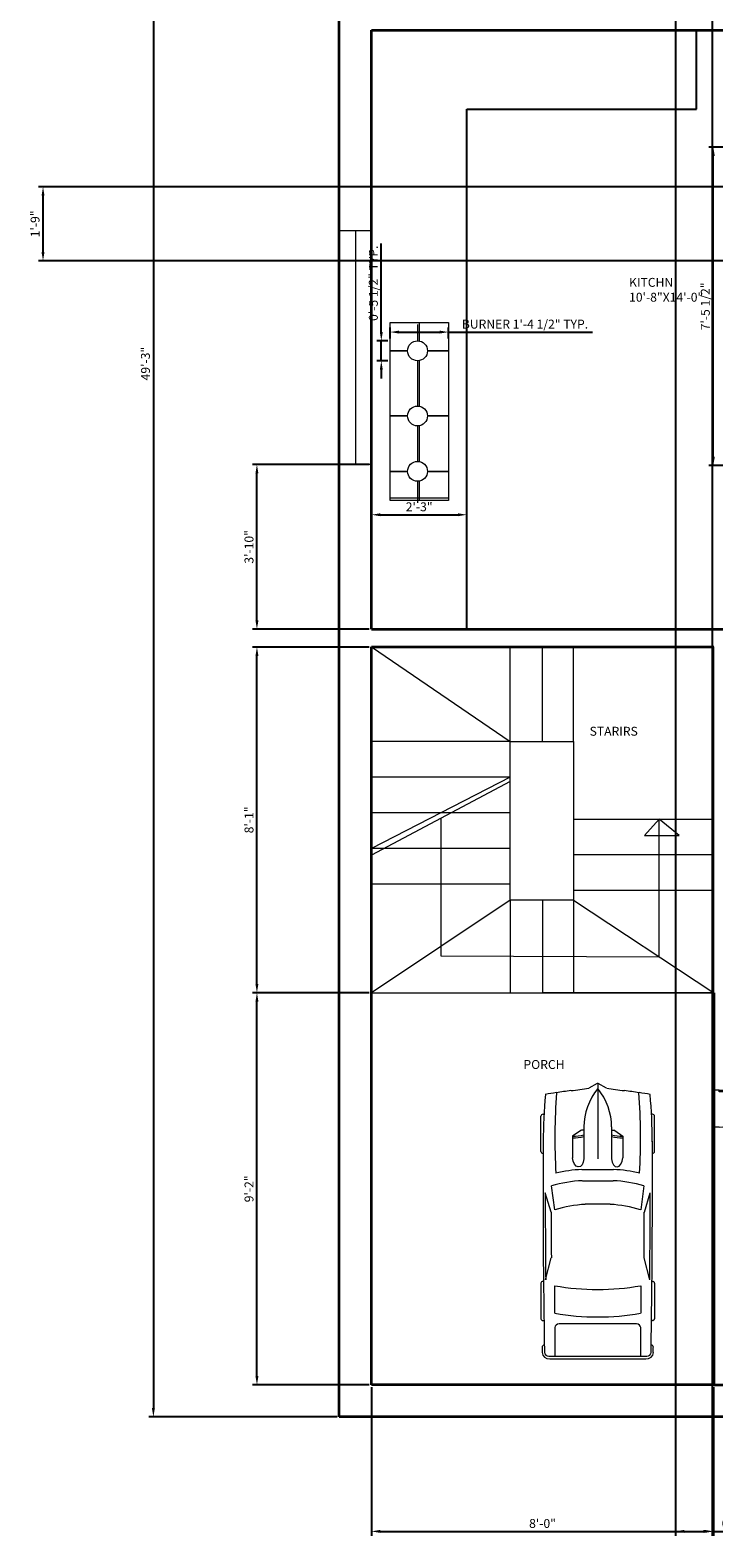
# Model space of a CAD drawing. Units: inches. Extents: x 311 to 793, y -3602 to -2932.
# Tile 1 of 3: x 313 to 505, y -3602 to -3179. Entities that reach past the tile are written whole.
import ezdxf

# ---------------------------------------------------------------- set-up
doc = ezdxf.new("R2010")
doc.units = ezdxf.units.IN
for name, color, linetype, lineweight in [('A-ANNO-DIMS', 2, 'Continuous', 18), ('A-AREA-IDEN', 7, 'Continuous', 18), ('A-DOOR', 3, 'Continuous', 18), ('A-EQPM', 9, 'Continuous', 18), ('A-FLOR-CASE', 9, 'Continuous', 25), ('A-FLOR-STRS', 7, 'Continuous', 18), ('A-GLAZ', 4, 'Continuous', 18), ('A-SITE-VEHC', 8, 'Continuous', 13), ('A-WALL', 7, 'Continuous', 35)]:
    doc.layers.add(name, color=color, linetype=linetype, lineweight=lineweight)
doc.styles.get("Standard").update_dxf_attribs({"font": 'arial.ttf'})
doc.dimstyles.new('ISO-25', dxfattribs={"dimtxt": 2.5, "dimasz": 2.5, "dimexe": 1.25, "dimexo": 0.625, "dimtad": 1, "dimlunit": 3, "dimtxsty": 'Standard', "dimcen": 2.5, "dimadec": 0, "dimazin": 0, "dimtfac": 1, "dimtmove": 0, "dimatfit": 3, "dimfxl": 1, "dimarcsym": 0})

# ---------------------------------------------------------------- blocks, each defined once
blk = doc.blocks.new('*U2')
for p, q in [((0, 0), (0, -6)), ((40, 0), (40, -6))]:
    blk.add_line(p, q)
blk.add_lwpolyline([(0, 0), (0, 40), (1.75, 40), (1.75, 0)], close=True)
blk.add_arc((0, 0), 40, 0, 90)
blk = doc.blocks.new('*U10')
for p, q in [((21.1, 37.4), (21.1, 36.8)), ((46.6, 38.9), (22.4, 38.9)), ((47.8, 37.4), (47.8, 37.4)), ((70, 31.5), (86.4, 29.4)), ((88, 31.9), (74.8, 35.9)), ((134.3, 35.6), (119.3, 31.8)), ((135.5, 37.1), (135.5, 37.4)), ((136.7, 38.9), (160.9, 38.9)), ((162.1, 37.4), (162.1, 36.8)), ((186.5, -33.5), (186.5, 33.5)), ((188.4, -32.8), (188.4, 32.8)), ((138.4, 29.4), (157.2, 29.4)), ((164.5, 26.4), (164.5, -26.4)), ((186.5, 29.4), (167, 29.4)), ((32.1, 9.5), (32.1, 11.2)), ((32.3, 11.6), (36.1, 17.2)), ((36.1, 17.2), (50.9, 17.2)), ((58.9, -10.8), (58.9, 10.8)), ((66.6, -10.5), (66.6, 10.5)), ((186.5, -10.5), (186.5, 10.5)), ((3.3, 6.1), (0.1, 0.4)), ((29.8, 9.5), (51.7, 9.5)), ((82.7, 8.5), (82.7, -8.5)), ((0, 0), (51.7, 0)), ((0.1, -0.4), (3.3, -6.1)), ((29.8, -9.5), (51.7, -9.5)), ((32.1, -9.5), (32.1, -11.2)), ((32.3, -11.6), (36.1, -17.2)), ((36.1, -17.2), (50.9, -17.2)), ((86.4, -29.4), (70, -31.5)), ((157.2, -29.4), (138.4, -29.4)), ((167, -29.4), (186.5, -29.4)), ((21.1, -37.4), (21.1, -36.8)), ((46.6, -38.9), (22.4, -38.9)), ((47.8, -37.4), (47.8, -37.4)), ((88, -31.9), (74.8, -35.9)), ((134.3, -35.6), (119.3, -31.8)), ((135.5, -37.1), (135.5, -37.4)), ((136.7, -38.9), (160.9, -38.9)), ((162.1, -37.4), (162.1, -36.8))]:
    blk.add_line(p, q)
for centre, major_axis, ratio, start_param, end_param in [((266, -27.5), (0, 313.3), 0.842304, 1.367076, 1.39176), ((41.2, -490.9), (0, 528.2), 0.842304, 0.00281, 0.075598), ((22.4, 37.4), (0, -1.48), 0.842304, 3.141593, 4.712389), ((64.5, -10555.6), (0, 10593), 0.842304, -0.013397, 0.002797), ((46.6, 37.4), (0, 1.48), 0.842304, -1.570796, 0), ((135.3, 5.4), (0, 81.8), 0.842304, 1.245306, 1.50788), ((64.5, -10555.6), (0, -10591.5), 0.842304, 3.133765, 3.140441), ((95.8, -3666.4), (0, -3698.2), 0.842304, 3.134049, 3.144098), ((136.7, 37.4), (0, -1.48), 0.842304, 3.141593, 4.712389), ((160.9, 37.4), (0, 1.48), 0.842304, -1.570796, 0), ((180.6, 35.8), (0, 2.22), 0.842304, -0.013017, 1.249894), ((64.5, -10556.4), (0, 10595.3), 0.842304, -0.013397, -0.013017), ((184, 32.8), (0, -5.25), 0.842304, 1.570796, 3.128196), ((184, 33.5), (0, -2.96), 0.842304, 1.570796, 3.128196), ((259.2, -27.5), (0, -305.3), 0.842304, 4.528606, 4.561838), ((37.5, -594), (0, -623.3), 0.842304, 3.096046, 3.200911), ((134.4, 5.4), (0, -89.8), 0.842304, 4.449482, 4.652344), ((149.6, 2.8), (0, -79.6), 0.842304, 4.372215, 4.640744), ((17.1, 0), (0, 147), 0.842304, 4.511394, 4.913384), ((35.9, 0), (0, 147), 0.842304, 4.511394, 4.913384), ((167, 26.4), (0, 2.96), 0.842304, 0, 1.570796), ((-204.5, 52.4), (0, -251), 0.842304, 1.385369, 1.434372), ((32.7, 11.2), (0, 0.74), 0.842304, 0.879714, 1.570796), ((13, 17), (0, 27.4), 0.842304, 4.435146, 4.718221), ((14.2, 17), (0, 27.4), 0.842304, 4.435146, 4.718221), ((50.8, 13.3), (6.34, -0.36), 0.603834, -1.395552, 1.581315), ((0.6, 0), (0, -0.74), 0.842304, 4.131459, 5.293319), ((29.8, -46.7), (0, 56.2), 0.842304, 0, 0.590319), ((-204.5, -52.4), (0, 251), 0.842304, -1.434372, -1.385369), ((29.8, 46.7), (0, 56.2), 0.842304, 2.551274, 3.141593), ((13, -17), (0, -27.4), 0.842304, 1.564964, 1.848039), ((14.2, -17), (0, -27.4), 0.842304, 1.564964, 1.848039), ((149.6, -2.8), (0, -79.6), 0.842304, -1.499151, -1.230623), ((259.2, 27.5), (0, 305.3), 0.842304, 1.721348, 1.754579), ((32.7, -11.2), (0, -0.74), 0.842304, 4.712389, 5.403472), ((134.4, -5.4), (0, -89.8), 0.842304, -1.510751, -1.307889), ((135.3, -5.4), (0, -81.8), 0.842304, -1.50788, -1.245306), ((266, 27.5), (0, 313.3), 0.842304, 1.749832, 1.774517), ((37.5, 594), (0, -623.3), 0.842304, -0.059319, 0.045547), ((167, -26.4), (0, -2.96), 0.842304, 4.712389, 6.283185), ((41.2, 490.9), (0, -528.2), 0.842304, -0.075598, -0.00281), ((22.4, -37.4), (0, 1.48), 0.842304, 1.570796, 3.141593), ((64.5, 10555.6), (0, 10593), 0.842304, 3.138796, 3.15499), ((46.6, -37.4), (0, -1.48), 0.842304, 0, 1.570796), ((64.5, 10555.6), (0, -10591.5), 0.842304, 0.001152, 0.007828), ((95.8, 3666.4), (0, -3698.2), 0.842304, -0.002505, 0.007544), ((136.7, -37.4), (0, -1.48), 0.842304, -1.570796, 0), ((160.9, -37.4), (0, 1.48), 0.842304, 3.141593, 4.712389), ((180.6, -35.8), (0, -2.22), 0.842304, -1.249894, 0.013017), ((64.5, 10556.4), (0, 10595.3), 0.842304, 3.15461, 3.15499), ((184, -32.8), (0, -5.25), 0.842304, 0.013397, 1.570796), ((184, -33.5), (0, 2.96), 0.842304, 3.15499, 4.712389)]:
    blk.add_ellipse(centre, major_axis=major_axis, ratio=ratio, start_param=start_param, end_param=end_param)
at = {"extrusion": (0, 0, -1)}
blk.add_ellipse((50.8, -13.3), major_axis=(6.34, 0.36), ratio=0.603834, start_param=-1.395552, end_param=1.581315, dxfattribs=at)
blk = doc.blocks.new('*D12')
at = {"layer": 'A-ANNO-DIMS', "color": 0, "lineweight": -2, "transparency": 16777216}
for p, q in [((399.17, -2976.63), (346.4, -2976.63)), ((347.65, -2979.13), (347.65, -3565.13)), ((399.17, -3567.63), (346.4, -3567.63))]:
    blk.add_line(p, q, dxfattribs=at)
at = {"layer": 'A-ANNO-DIMS', "color": 0, "transparency": 16777216}
for points in [[(347.23, -2979.13), (348.07, -2979.13), (347.65, -2976.63)], [(347.23, -3565.13), (348.07, -3565.13), (347.65, -3567.63)]]:
    blk.add_solid(points, dxfattribs=at)
at = {"layer": 'Defpoints', "color": 0, "transparency": 16777216}
for p in [(399.79, -2976.63), (347.65, -3567.63), (399.79, -3567.63)]:
    blk.add_point(p, dxfattribs=at)
at = {"layer": 'A-ANNO-DIMS', "color": 0, "transparency": 16777216, "insert": (345.75, -3272.13), "char_height": 2.5, "attachment_point": 5, "rotation": 90}
blk.add_mtext('49\'-3"', dxfattribs=at)
blk = doc.blocks.new('WINDOW-SIDE-66')
for p, q in [((0, 65.66), (9, 65.66)), ((0, 0), (0, 65.66)), ((0, 65.66), (4.5, 65.66)), ((4.5, 65.66), (4.5, 0)), ((9, 65.66), (9, 0)), ((9, 0), (0, 0))]:
    blk.add_line(p, q)
blk = doc.blocks.new('COOKTOP-BURNER')
for p, q in [((4.91, 2.79), (0, 2.79)), ((4.91, 2.69), (0, 2.69)), ((16.38, 2.79), (10.5, 2.79)), ((10.5, 2.79), (16.38, 2.79)), ((16.38, 2.69), (10.5, 2.69))]:
    blk.add_line(p, q)
blk.add_circle((7.71, 2.79), 2.79)
blk = doc.blocks.new('*D20')
at = {"layer": 'A-ANNO-DIMS', "color": 0, "lineweight": -2, "transparency": 16777216}
for p, q in [((414.03, -3265.11), (414.03, -3262.03)), ((416.53, -3263.28), (427.91, -3263.28)), ((430.41, -3265.11), (430.41, -3262.03)), ((430.41, -3263.28), (470.83, -3263.28))]:
    blk.add_line(p, q, dxfattribs=at)
at = {"layer": 'A-ANNO-DIMS', "color": 0, "transparency": 16777216}
for points in [[(416.53, -3262.87), (416.53, -3263.7), (414.03, -3263.28)], [(427.91, -3262.87), (427.91, -3263.7), (430.41, -3263.28)]]:
    blk.add_solid(points, dxfattribs=at)
at = {"layer": 'Defpoints', "color": 0, "transparency": 16777216}
for p in [(430.41, -3263.28), (414.03, -3265.74), (430.41, -3265.74)]:
    blk.add_point(p, dxfattribs=at)
at = {"layer": 'A-ANNO-DIMS', "color": 0, "transparency": 16777216, "insert": (451.87, -3261.37), "char_height": 2.5, "attachment_point": 5}
blk.add_mtext('BURNER 1\'-4 1/2" TYP.', dxfattribs=at)
blk = doc.blocks.new('*D21')
at = {"layer": 'A-ANNO-DIMS', "color": 0, "lineweight": -2, "transparency": 16777216}
for p, q in [((411.57, -3263.24), (411.57, -3238.43)), ((413.4, -3265.74), (410.32, -3265.74)), ((411.57, -3271.32), (411.57, -3265.74)), ((413.4, -3271.32), (410.32, -3271.32)), ((411.57, -3273.82), (411.57, -3276.32))]:
    blk.add_line(p, q, dxfattribs=at)
at = {"layer": 'A-ANNO-DIMS', "color": 0, "transparency": 16777216}
for points in [[(411.16, -3263.24), (411.99, -3263.24), (411.57, -3265.74)], [(411.16, -3273.82), (411.99, -3273.82), (411.57, -3271.32)]]:
    blk.add_solid(points, dxfattribs=at)
at = {"layer": 'Defpoints', "color": 0, "transparency": 16777216}
for p in [(411.57, -3265.74), (414.03, -3265.74), (414.03, -3271.32)]:
    blk.add_point(p, dxfattribs=at)
at = {"layer": 'A-ANNO-DIMS', "color": 0, "transparency": 16777216, "insert": (409.66, -3249.58), "char_height": 2.5, "attachment_point": 5, "rotation": 90}
blk.add_mtext('0\'-5 1/2" TYP.', dxfattribs=at)
blk = doc.blocks.new('*D25')
at = {"layer": 'A-ANNO-DIMS', "color": 0, "lineweight": -2, "transparency": 16777216}
for p, q in [((408.79, -3559.25), (408.79, -3600.98)), ((504.79, -3559.25), (504.79, -3600.98)), ((411.29, -3599.73), (502.29, -3599.73))]:
    blk.add_line(p, q, dxfattribs=at)
at = {"layer": 'A-ANNO-DIMS', "color": 0, "transparency": 16777216}
for points in [[(411.29, -3599.31), (411.29, -3600.14), (408.79, -3599.73)], [(502.29, -3599.31), (502.29, -3600.14), (504.79, -3599.73)]]:
    blk.add_solid(points, dxfattribs=at)
at = {"layer": 'Defpoints', "color": 0, "transparency": 16777216}
for p in [(408.79, -3558.63), (504.79, -3558.63), (504.79, -3599.73)]:
    blk.add_point(p, dxfattribs=at)
at = {"layer": 'A-ANNO-DIMS', "color": 0, "transparency": 16777216, "insert": (456.79, -3597.82), "char_height": 2.5, "attachment_point": 5}
blk.add_mtext('8\'-0"', dxfattribs=at)
blk = doc.blocks.new('*D32')
at = {"layer": 'A-ANNO-DIMS', "color": 0, "lineweight": -2, "transparency": 16777216}
for p, q in [((408.17, -3448.63), (375.44, -3448.63)), ((376.69, -3556.13), (376.69, -3451.13)), ((408.17, -3558.63), (375.44, -3558.63))]:
    blk.add_line(p, q, dxfattribs=at)
at = {"layer": 'A-ANNO-DIMS', "color": 0, "transparency": 16777216}
for points in [[(376.27, -3451.13), (377.11, -3451.13), (376.69, -3448.63)], [(376.27, -3556.13), (377.11, -3556.13), (376.69, -3558.63)]]:
    blk.add_solid(points, dxfattribs=at)
at = {"layer": 'Defpoints', "color": 0, "transparency": 16777216}
for p in [(376.69, -3448.63), (408.79, -3448.63), (408.79, -3558.63)]:
    blk.add_point(p, dxfattribs=at)
at = {"layer": 'A-ANNO-DIMS', "color": 0, "transparency": 16777216, "insert": (374.79, -3503.63), "char_height": 2.5, "attachment_point": 5, "rotation": 90}
blk.add_mtext('9\'-2"', dxfattribs=at)
blk = doc.blocks.new('*D33')
at = {"layer": 'A-ANNO-DIMS', "color": 0, "lineweight": -2, "transparency": 16777216}
for p, q in [((408.17, -3351.63), (375.44, -3351.63)), ((376.69, -3446.13), (376.69, -3354.13)), ((408.17, -3448.63), (375.44, -3448.63))]:
    blk.add_line(p, q, dxfattribs=at)
at = {"layer": 'A-ANNO-DIMS', "color": 0, "transparency": 16777216}
for points in [[(376.27, -3354.13), (377.11, -3354.13), (376.69, -3351.63)], [(376.27, -3446.13), (377.11, -3446.13), (376.69, -3448.63)]]:
    blk.add_solid(points, dxfattribs=at)
at = {"layer": 'Defpoints', "color": 0, "transparency": 16777216}
for p in [(376.69, -3351.63), (408.79, -3351.63), (408.79, -3448.63)]:
    blk.add_point(p, dxfattribs=at)
at = {"layer": 'A-ANNO-DIMS', "color": 0, "transparency": 16777216, "insert": (374.79, -3400.13), "char_height": 2.5, "attachment_point": 5, "rotation": 90}
blk.add_mtext('8\'-1"', dxfattribs=at)
blk = doc.blocks.new('*D43')
at = {"layer": 'A-ANNO-DIMS', "color": 0, "lineweight": -2, "transparency": 16777216}
for p, q in [((408.17, -3300.45), (375.44, -3300.45)), ((376.69, -3344.13), (376.69, -3302.95)), ((408.17, -3346.63), (375.44, -3346.63))]:
    blk.add_line(p, q, dxfattribs=at)
at = {"layer": 'A-ANNO-DIMS', "color": 0, "transparency": 16777216}
for points in [[(376.27, -3302.95), (377.11, -3302.95), (376.69, -3300.45)], [(376.27, -3344.13), (377.11, -3344.13), (376.69, -3346.63)]]:
    blk.add_solid(points, dxfattribs=at)
at = {"layer": 'Defpoints', "color": 0, "transparency": 16777216}
for p in [(376.69, -3300.45), (408.79, -3300.45), (408.79, -3346.63)]:
    blk.add_point(p, dxfattribs=at)
at = {"layer": 'A-ANNO-DIMS', "color": 0, "transparency": 16777216, "insert": (374.79, -3323.54), "char_height": 2.5, "attachment_point": 5, "rotation": 90}
blk.add_mtext('3\'-10"', dxfattribs=at)
blk = doc.blocks.new('*D46')
at = {"layer": 'A-ANNO-DIMS', "color": 0, "lineweight": -2, "transparency": 16777216}
for p, q in [((591.8, -3222.54), (315.44, -3222.54)), ((316.69, -3240.8), (316.69, -3225.04)), ((591.8, -3243.3), (315.44, -3243.3))]:
    blk.add_line(p, q, dxfattribs=at)
at = {"layer": 'A-ANNO-DIMS', "color": 0, "transparency": 16777216}
for points in [[(316.27, -3225.04), (317.11, -3225.04), (316.69, -3222.54)], [(316.27, -3240.8), (317.11, -3240.8), (316.69, -3243.3)]]:
    blk.add_solid(points, dxfattribs=at)
at = {"layer": 'Defpoints', "color": 0, "transparency": 16777216}
for p in [(316.69, -3222.54), (592.43, -3222.54), (592.43, -3243.3)]:
    blk.add_point(p, dxfattribs=at)
at = {"layer": 'A-ANNO-DIMS', "color": 0, "transparency": 16777216, "insert": (314.79, -3232.92), "char_height": 2.5, "attachment_point": 5, "rotation": 90}
blk.add_mtext('1\'-9"', dxfattribs=at)
blk = doc.blocks.new('*D50')
at = {"layer": 'A-ANNO-DIMS', "color": 0, "lineweight": -2, "transparency": 16777216}
for p, q in [((494.06, -3042.22), (494.06, -3600.98)), ((504.38, -3042.22), (504.38, -3600.98)), ((496.56, -3599.73), (501.88, -3599.73)), ((504.38, -3599.73), (522.54, -3599.73))]:
    blk.add_line(p, q, dxfattribs=at)
at = {"layer": 'A-ANNO-DIMS', "color": 0, "transparency": 16777216}
for points in [[(496.56, -3599.31), (496.56, -3600.14), (494.06, -3599.73)], [(501.88, -3599.31), (501.88, -3600.14), (504.38, -3599.73)]]:
    blk.add_solid(points, dxfattribs=at)
at = {"layer": 'Defpoints', "color": 0, "transparency": 16777216}
for p in [(494.06, -3041.59), (504.38, -3041.59), (504.38, -3599.73)]:
    blk.add_point(p, dxfattribs=at)
at = {"layer": 'A-ANNO-DIMS', "color": 0, "transparency": 16777216, "insert": (514.71, -3597.81), "char_height": 2.5, "attachment_point": 5}
blk.add_mtext('0\'-10 1/2"', dxfattribs=at)
blk = doc.blocks.new('*D51')
at = {"layer": 'A-ANNO-DIMS', "color": 0, "lineweight": -2, "transparency": 16777216}
for p, q in [((408.79, -3346), (408.79, -3313.28)), ((411.29, -3314.53), (433.1, -3314.53)), ((435.6, -3346), (435.6, -3313.28))]:
    blk.add_line(p, q, dxfattribs=at)
at = {"layer": 'A-ANNO-DIMS', "color": 0, "transparency": 16777216}
for points in [[(411.29, -3314.11), (411.29, -3314.94), (408.79, -3314.53)], [(433.1, -3314.11), (433.1, -3314.94), (435.6, -3314.53)]]:
    blk.add_solid(points, dxfattribs=at)
at = {"layer": 'Defpoints', "color": 0, "transparency": 16777216}
for p in [(435.6, -3314.53), (408.79, -3346.63), (435.6, -3346.63)]:
    blk.add_point(p, dxfattribs=at)
at = {"layer": 'A-ANNO-DIMS', "color": 0, "transparency": 16777216, "insert": (422.2, -3312.62), "char_height": 2.5, "attachment_point": 5}
blk.add_mtext('2\'-3"', dxfattribs=at)
blk = doc.blocks.new('*D53')
at = {"layer": 'A-ANNO-DIMS', "color": 0, "lineweight": -2, "transparency": 16777216}
for p, q in [((536.17, -3211.42), (503.44, -3211.42)), ((504.69, -3298.24), (504.69, -3213.92)), ((536.17, -3300.74), (503.44, -3300.74))]:
    blk.add_line(p, q, dxfattribs=at)
at = {"layer": 'A-ANNO-DIMS', "color": 0, "transparency": 16777216}
for points in [[(504.27, -3213.92), (505.11, -3213.92), (504.69, -3211.42)], [(504.27, -3298.24), (505.11, -3298.24), (504.69, -3300.74)]]:
    blk.add_solid(points, dxfattribs=at)
at = {"layer": 'Defpoints', "color": 0, "transparency": 16777216}
for p in [(504.69, -3211.42), (536.79, -3211.42), (536.79, -3300.74)]:
    blk.add_point(p, dxfattribs=at)
at = {"layer": 'A-ANNO-DIMS', "color": 0, "transparency": 16777216, "insert": (502.77, -3256.08), "char_height": 2.5, "attachment_point": 5, "rotation": 90}
blk.add_mtext('7\'-5 1/2"', dxfattribs=at)

msp = doc.modelspace()

# ---------------------------------------------------------------- linework, layer by layer
at = {"layer": 'A-EQPM'}
for p, q in [((422.217, -3260.551), (422.217, -3265.782)), ((421.734, -3261.138), (421.734, -3265.74)), ((421.734, -3271.324), (421.734, -3284.021)), ((422.217, -3271.282), (422.217, -3284.063)), ((421.734, -3289.605), (421.734, -3299.556)), ((422.217, -3289.563), (422.217, -3299.598)), ((421.734, -3305.14), (421.734, -3311.157)), ((422.217, -3305.098), (422.217, -3310.569)), ((430.405, -3309.848), (414.029, -3309.848))]:
    msp.add_line(p, q, dxfattribs=at)
msp.add_lwpolyline([(414.029, -3260.551), (430.405, -3260.551), (430.405, -3310.569), (414.029, -3310.569)], close=True, dxfattribs=at)
at = {"layer": 'A-FLOR-CASE'}
for p, q in [((499.979, -3200.763), (499.979, -3178.626)), ((435.603, -3346.626), (435.603, -3200.763)), ((435.603, -3200.763), (499.979, -3200.763))]:
    msp.add_line(p, q, dxfattribs=at)
at = {"layer": 'A-FLOR-STRS'}
for p, q in [((408.791, -3351.626), (408.791, -3448.626)), ((408.791, -3351.626), (447.725, -3378.123)), ((447.725, -3378.123), (447.725, -3351.626)), ((456.791, -3378.123), (456.791, -3351.626)), ((456.791, -3378.123), (456.791, -3351.626)), ((465.491, -3378.123), (465.491, -3351.626)), ((504.791, -3448.626), (504.791, -3351.626)), ((447.725, -3378.123), (408.791, -3378.123)), ((447.725, -3388.123), (408.791, -3388.123)), ((447.725, -3388.123), (408.791, -3408.123)), ((447.725, -3389.317), (408.791, -3409.981)), ((447.725, -3398.123), (408.791, -3398.123)), ((428.258, -3399.649), (428.258, -3438.302)), ((465.491, -3399.882), (504.791, -3399.882)), ((489.538, -3399.882), (485.421, -3404.539)), ((489.538, -3438.543), (489.538, -3399.882)), ((495.115, -3404.539), (489.538, -3399.882)), ((485.421, -3404.539), (495.115, -3404.539)), ((447.725, -3408.123), (408.791, -3408.123)), ((465.491, -3409.882), (504.791, -3409.882)), ((447.725, -3418.123), (408.791, -3418.123)), ((465.491, -3419.882), (504.791, -3419.882)), ((447.725, -3422.648), (408.791, -3448.626)), ((447.725, -3422.648), (447.725, -3448.626)), ((456.791, -3422.648), (456.791, -3448.626)), ((465.491, -3422.648), (465.491, -3448.626)), ((465.491, -3422.648), (504.791, -3448.626)), ((428.258, -3438.302), (489.538, -3438.543)), ((408.791, -3448.626), (504.791, -3448.626)), ((408.791, -3448.626), (456.791, -3448.626)), ((408.791, -3448.626), (456.791, -3448.626)), ((504.791, -3448.626), (456.791, -3448.626)), ((504.791, -3448.626), (456.791, -3448.626)), ((504.791, -3448.626), (456.791, -3448.626)), ((504.791, -3448.626), (456.791, -3448.626))]:
    msp.add_line(p, q, dxfattribs=at)
msp.add_lwpolyline([(447.725, -3378.123), (465.491, -3378.123), (465.491, -3422.648), (447.725, -3422.648)], close=True, dxfattribs=at)
at = {"layer": 'A-WALL'}
for p, q in [((399.791, -3567.626), (399.791, -2967.626)), ((408.791, -3178.626), (536.791, -3178.626)), ((408.791, -3346.626), (408.791, -3178.626)), ((408.791, -3346.626), (408.791, -3338.626)), ((408.791, -3346.626), (536.791, -3346.626)), ((408.791, -3558.626), (408.791, -3351.626)), ((408.791, -3351.626), (504.791, -3351.626)), ((408.791, -3558.626), (408.791, -3351.626)), ((504.791, -3448.626), (504.791, -3558.626)), ((504.791, -3558.626), (408.791, -3558.626)), ((504.791, -3558.626), (599.791, -3558.626)), ((759.791, -3567.626), (399.791, -3567.626))]:
    msp.add_line(p, q, dxfattribs=at)

# ---------------------------------------------------------------- block references
at = {"layer": 'A-DOOR', "xscale": 0.2580993088148874, "yscale": 0.2580993088148874, "zscale": 0.2580993088148874, "rotation": 270}
msp.add_blockref('*U2', (506.298, -3475.99), dxfattribs=at)
at = {"layer": 'A-EQPM'}
for p in [(414.029, -3271.324), (414.029, -3289.605), (414.029, -3305.14)]:
    msp.add_blockref('COOKTOP-BURNER', p, dxfattribs=at)
at = {"layer": 'A-GLAZ'}
msp.add_blockref('WINDOW-SIDE-66', (399.791, -3300.454), dxfattribs=at)
at = {"layer": 'A-SITE-VEHC', "xscale": 0.4102453860597914, "yscale": 0.4102453860597914, "zscale": 0.4102453860597914, "rotation": 270}
msp.add_blockref('*U10', (472.272, -3474.043), dxfattribs=at)

# ---------------------------------------------------------------- texts
at = {"layer": 'A-AREA-IDEN', "char_height": 2.5, "attachment_point": 1}
for s, width, insert in [('KITCHN\\P10\'-8"X14\'-0"', 67.49127, (481.068, -3248.089)), ('STARIRS', 25.57194, (469.998, -3374.014)), ('PORCH', 33.95667, (451.448, -3467.499))]:
    msp.add_mtext_dynamic_manual_height_columns(s, width=width, gutter_width=12.5, heights=[0], dxfattribs=dict(at, insert=insert))

# ---------------------------------------------------------------- dimensions: what is measured, and where the dimension line sits
at = {"layer": 'A-ANNO-DIMS'}
for base, p1, p2, override, picture, middle in [((347.649, -3567.626), (399.791, -2976.626), (399.791, -3567.626), {"dimclrd": 0, "dimclre": 0, "dimclrt": 0}, '*D12', (345.746, -3272.126)), ((504.691, -3211.417), (536.791, -3300.744), (536.791, -3211.417), {"dimdec": 1, "dimlfac": 1, "dimrnd": 0, "dimzin": 1, "dimdsep": 46, "dimlunit": 4, "dimfrac": 2}, '*D53', (502.773, -3256.08)), ((316.691, -3222.538), (592.429, -3243.296), (592.429, -3222.538), {"dimdec": 1, "dimlfac": 1, "dimrnd": 0, "dimzin": 1, "dimdsep": 46, "dimlunit": 4, "dimfrac": 2}, '*D46', (314.79, -3232.917)), ((376.691, -3300.454), (408.791, -3346.626), (408.791, -3300.454), {"dimdec": 1, "dimlfac": 1, "dimrnd": 0, "dimzin": 1, "dimdsep": 46, "dimlunit": 4, "dimfrac": 2}, '*D43', (374.789, -3323.54)), ((376.691, -3351.626), (408.791, -3448.626), (408.791, -3351.626), {"dimdec": 1, "dimlfac": 1, "dimrnd": 0, "dimzin": 1, "dimdsep": 46, "dimlunit": 4, "dimfrac": 2}, '*D33', (374.79, -3400.126)), ((376.691, -3448.626), (408.791, -3558.626), (408.791, -3448.626), {"dimdec": 1, "dimlfac": 1, "dimrnd": 0, "dimzin": 1, "dimdsep": 46, "dimlunit": 4, "dimfrac": 2}, '*D32', (374.79, -3503.626))]:
    dim = msp.add_linear_dim(base=base, p1=p1, p2=p2, angle=90, dimstyle='ISO-25', override=override, dxfattribs=at)
    dim.commit()
    dim.dimension.update_dxf_attribs({"geometry": picture, "text_midpoint": middle})
for base, p1, p2, picture, middle in [((504.381, -3599.726), (494.057, -3041.593), (504.381, -3041.593), '*D50', (514.712, -3597.808)), ((435.603, -3314.526), (408.791, -3346.626), (435.603, -3346.626), '*D51', (422.197, -3312.623)), ((504.791, -3599.726), (408.791, -3558.626), (504.791, -3558.626), '*D25', (456.791, -3597.824))]:
    dim = msp.add_linear_dim(base=base, p1=p1, p2=p2, dimstyle='ISO-25', override={"dimdec": 1, "dimlfac": 1, "dimrnd": 0, "dimzin": 1, "dimdsep": 46, "dimlunit": 4, "dimfrac": 2}, dxfattribs=at)
    dim.commit()
    dim.dimension.update_dxf_attribs({"geometry": picture, "text_midpoint": middle})
dim = msp.add_linear_dim(base=(411.573, -3265.74), p1=(414.029, -3271.324), p2=(414.029, -3265.74), angle=90, text='<> TYP.', dimstyle='ISO-25', override={"dimdec": 1, "dimlfac": 1, "dimrnd": 0, "dimzin": 1, "dimdsep": 46, "dimlunit": 4, "dimfrac": 2}, dxfattribs=at)
dim.commit()
dim.dimension.update_dxf_attribs({"geometry": '*D21', "text_midpoint": (409.655, -3249.583)})
dim = msp.add_linear_dim(base=(430.405, -3263.283), p1=(414.029, -3265.74), p2=(430.405, -3265.74), text='BURNER <> TYP.', dimstyle='ISO-25', override={"dimdec": 1, "dimlfac": 1, "dimrnd": 0, "dimzin": 1, "dimdsep": 46, "dimlunit": 4, "dimfrac": 2}, dxfattribs=at)
dim.commit()
dim.dimension.update_dxf_attribs({"geometry": '*D20', "text_midpoint": (451.866, -3261.366)})

doc.saveas('drawing.dxf')
